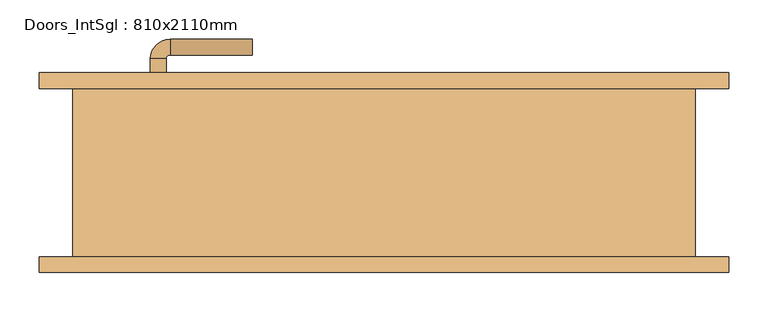
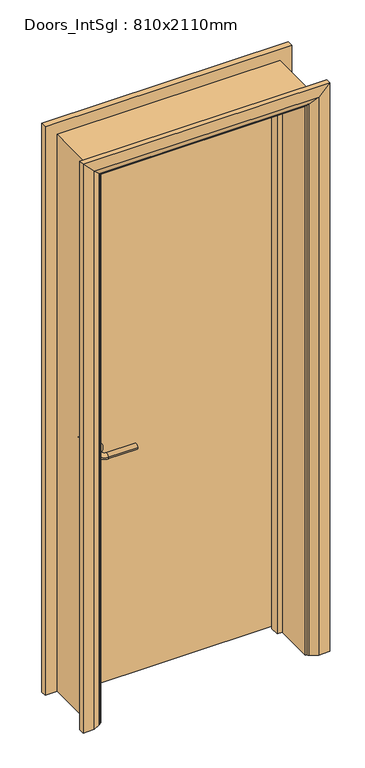
"""IFC4 building model written with IfcOpenShell, lengths in millimetres: door geometry, Doors_IntSgl : 810x2110mm."""

from ifc_helpers import new_model, si_unit, point, frame, frame_2d, origin, place, context, project, spatial, polyline, circle_curve, ellipse_curve, trimmed, segment, composite_curve, outline, extrude, faceted_brep, source, transform, mapped, element, save
from ifc_brep_helpers import plane_surface, cylinder_surface, revolved_surface, advanced_brep


def doors_intsgl_810x2110mm_df607d29(model_context):
    return source(origin(), model_context, "Body", "SolidModel", [
        advanced_brep(
        [(-298.0, 61.5, 900.0), (-278.0, 61.5, 900.0), (-278.0, 31.5, 900.0), (-298.0, 31.5, 900.0), (-273.0, 26.5, 900.0), (-273.0, 6.5, 900.0), (-168.0, 6.5, 900.0), (-168.0, 26.5, 900.0)],
        [
            (0, 1, circle_curve(frame((-288.0, 61.5, 900.0), z_axis=(0.0, 1.0, 0.0), x_axis=(1.0, 0.0, 0.0)), 10.0)),
            (1, 0, circle_curve(frame((-288.0, 61.5, 900.0), z_axis=(0.0, 1.0, 0.0), x_axis=(1.0, 0.0, 0.0)), 10.0)),
            (1, 2),
            (2, 3, circle_curve(frame((-288.0, 31.5, 900.0), z_axis=(0.0, 1.0, 0.0), x_axis=(1.0, 0.0, 0.0)), 10.0)),
            (3, 0),
            (3, 2, circle_curve(frame((-288.0, 31.5, 900.0), z_axis=(0.0, 1.0, 0.0), x_axis=(1.0, 0.0, 0.0)), 10.0)),
            (4, 5, circle_curve(frame((-273.0, 16.5, 900.0), z_axis=(-1.0, 0.0, 0.0), x_axis=(0.0, 1.0, 0.0)), 10.0)),
            (5, 3, circle_curve(frame((-273.0, 31.5, 900.0), z_axis=(0.0, 0.0, -1.0), x_axis=(-1.0, 0.0, 0.0)), 25.0)),
            (2, 4, circle_curve(frame((-273.0, 31.5, 900.0), z_axis=(0.0, 0.0, 1.0), x_axis=(-1.0, 0.0, 0.0)), 5.0)),
            (5, 4, circle_curve(frame((-273.0, 16.5, 900.0), z_axis=(-1.0, 0.0, 0.0), x_axis=(0.0, 1.0, 0.0)), 10.0)),
            (6, 7, circle_curve(frame((-168.0, 16.5, 900.0), z_axis=(1.0, 0.0, 0.0), x_axis=(0.0, 1.0, 0.0)), 10.0)),
            (7, 6, circle_curve(frame((-168.0, 16.5, 900.0), z_axis=(1.0, 0.0, 0.0), x_axis=(0.0, 1.0, 0.0)), 10.0)),
            (4, 7),
            (6, 5),
        ],
        [
            plane_surface(frame((-288.0, 61.5, 900.0), z_axis=(0.0, 1.0, 0.0), x_axis=(0.0, 0.0, 1.0))),
            cylinder_surface(frame((-288.0, 61.5, 900.0), z_axis=(0.0, 1.0, 0.0), x_axis=(1.0, 0.0, 0.0)), 10.0),
            revolved_surface(trimmed(ellipse_curve(frame((-288.0, 31.5, 900.0), z_axis=(0.0, -1.0, 0.0), x_axis=(1.0, 0.0, 0.0)), 10.0, 10.0), [point((-298.0, 31.5, 900.0))], [point((-278.0, 31.5, 900.0))], True, "CARTESIAN"), (-273.0, 31.5, 900.0), (0.0, 0.0, -1.0)),
            revolved_surface(trimmed(ellipse_curve(frame((-288.0, 31.5, 900.0), z_axis=(0.0, -1.0, 0.0), x_axis=(1.0, 0.0, 0.0)), 10.0, 10.0), [point((-278.0, 31.5, 900.0))], [point((-298.0, 31.5, 900.0))], True, "CARTESIAN"), (-273.0, 31.5, 900.0), (0.0, 0.0, -1.0)),
            plane_surface(frame((-168.0, 16.5, 900.0), z_axis=(1.0, 0.0, 0.0), x_axis=(0.0, 0.0, 1.0))),
            cylinder_surface(frame((-273.0, 16.5, 900.0), z_axis=(-1.0, 0.0, 0.0), x_axis=(0.0, 1.0, 0.0)), 10.0),
        ],
        [
            (0, [[1, 2]]),
            (1, [[3, 4, 5, -2]]),
            (1, [[-5, 6, -3, -1]]),
            (2, [[7, 8, -4, 9]]),
            (3, [[10, -9, -6, -8]]),
            (4, [[11, 12]]),
            (5, [[13, -11, 14, -7]]),
            (5, [[-14, -12, -13, -10]]),
        ],
    ),
        extrude(outline(composite_curve([segment(trimmed(circle_curve(frame_2d((900.0, -290.5)), 30.0), [point((900.0, -320.5))], [point((900.0, -260.5))], False, "CARTESIAN"), True, "CONTINUOUS"), segment(trimmed(circle_curve(frame_2d((900.0, -290.5)), 30.0), [point((900.0, -260.5))], [point((900.0, -320.5))], False, "CARTESIAN"), True, "CONTINUOUS")], self_intersect=False)), frame((0.0, 61.5, 0.0), z_axis=(0.0, 1.0, 0.0), x_axis=(0.0, 0.0, 1.0)), (0.0, 0.0, 1.0), 8.0),
        advanced_brep(
        [(-298.0, 115.5, 900.0), (-278.0, 115.5, 900.0), (-298.0, 145.5, 900.0), (-278.0, 145.5, 900.0), (-273.0, 150.5, 900.0), (-273.0, 170.5, 900.0), (-168.0, 170.5, 900.0), (-168.0, 150.5, 900.0)],
        [
            (0, 1, circle_curve(frame((-288.0, 115.5, 900.0), z_axis=(0.0, -1.0, 0.0), x_axis=(1.0, 0.0, 0.0)), 10.0)),
            (1, 0, circle_curve(frame((-288.0, 115.5, 900.0), z_axis=(0.0, -1.0, 0.0), x_axis=(1.0, 0.0, 0.0)), 10.0)),
            (0, 2),
            (2, 3, circle_curve(frame((-288.0, 145.5, 900.0), z_axis=(0.0, -1.0, 0.0), x_axis=(1.0, 0.0, 0.0)), 10.0)),
            (3, 1),
            (3, 2, circle_curve(frame((-288.0, 145.5, 900.0), z_axis=(0.0, -1.0, 0.0), x_axis=(1.0, 0.0, 0.0)), 10.0)),
            (4, 3, circle_curve(frame((-273.0, 145.5, 900.0), z_axis=(0.0, 0.0, 1.0), x_axis=(-1.0, 0.0, 0.0)), 5.0)),
            (2, 5, circle_curve(frame((-273.0, 145.5, 900.0), z_axis=(0.0, 0.0, -1.0), x_axis=(-1.0, 0.0, 0.0)), 25.0)),
            (5, 4, circle_curve(frame((-273.0, 160.5, 900.0), z_axis=(-1.0, 0.0, 0.0), x_axis=(0.0, -1.0, 0.0)), 10.0)),
            (4, 5, circle_curve(frame((-273.0, 160.5, 900.0), z_axis=(-1.0, 0.0, 0.0), x_axis=(0.0, -1.0, 0.0)), 10.0)),
            (6, 7, circle_curve(frame((-168.0, 160.5, 900.0), z_axis=(1.0, 0.0, 0.0), x_axis=(0.0, -1.0, 0.0)), 10.0)),
            (7, 6, circle_curve(frame((-168.0, 160.5, 900.0), z_axis=(1.0, 0.0, 0.0), x_axis=(0.0, -1.0, 0.0)), 10.0)),
            (5, 6),
            (7, 4),
        ],
        [
            plane_surface(frame((-288.0, 115.5, 900.0), z_axis=(0.0, -1.0, 0.0), x_axis=(0.0, 0.0, 1.0))),
            cylinder_surface(frame((-288.0, 115.5, 900.0), z_axis=(0.0, -1.0, 0.0), x_axis=(1.0, 0.0, 0.0)), 10.0),
            revolved_surface(trimmed(ellipse_curve(frame((-288.0, 145.5, 900.0), z_axis=(0.0, -1.0, 0.0), x_axis=(1.0, 0.0, 0.0)), 10.0, 10.0), [point((-298.0, 145.5, 900.0))], [point((-278.0, 145.5, 900.0))], True, "CARTESIAN"), (-273.0, 145.5, 900.0), (0.0, 0.0, -1.0)),
            revolved_surface(trimmed(ellipse_curve(frame((-288.0, 145.5, 900.0), z_axis=(0.0, -1.0, 0.0), x_axis=(1.0, 0.0, 0.0)), 10.0, 10.0), [point((-278.0, 145.5, 900.0))], [point((-298.0, 145.5, 900.0))], True, "CARTESIAN"), (-273.0, 145.5, 900.0), (0.0, 0.0, -1.0)),
            plane_surface(frame((-168.0, 160.5, 900.0), z_axis=(1.0, 0.0, 0.0), x_axis=(0.0, 0.0, 1.0))),
            cylinder_surface(frame((-273.0, 160.5, 900.0), z_axis=(-1.0, 0.0, 0.0), x_axis=(0.0, -1.0, 0.0)), 10.0),
        ],
        [
            (0, [[1, 2]]),
            (1, [[-1, 3, 4, 5]]),
            (1, [[-2, -5, 6, -3]]),
            (2, [[7, -4, 8, 9]]),
            (3, [[-8, -6, -7, 10]]),
            (4, [[11, 12]]),
            (5, [[-9, 13, -12, 14]]),
            (5, [[-10, -14, -11, -13]]),
        ],
    ),
        extrude(outline(composite_curve([segment(trimmed(circle_curve(frame_2d((900.0, -290.5)), 30.0), [point((900.0, -320.5))], [point((900.0, -260.5))], False, "CARTESIAN"), True, "CONTINUOUS"), segment(trimmed(circle_curve(frame_2d((900.0, -290.5)), 30.0), [point((900.0, -260.5))], [point((900.0, -320.5))], False, "CARTESIAN"), True, "CONTINUOUS")], self_intersect=False)), frame((0.0, 107.5, 0.0), z_axis=(0.0, 1.0, 0.0), x_axis=(0.0, 0.0, 1.0)), (0.0, 0.0, 1.0), 8.0),
        extrude(outline(polyline([(363.0, 69.5), (-363.0, 69.5), (-363.0, 107.5), (363.0, 107.5), (363.0, 69.5)])), frame((0.0, 0.0, 8.0), z_axis=(0.0, 0.0, 1.0), x_axis=(1.0, 0.0, 0.0)), (0.0, 0.0, 1.0), 2060.0),
        advanced_brep(
        [(440.0, 127.5, 0.0), (440.0, 107.5, 0.0), (370.0, 107.5, 0.0), (374.0, 113.5, 0.0), (400.0, 127.5, 0.0), (440.0, 127.5, 2145.0), (440.0, 107.5, 2145.0), (-440.0, 107.5, 2145.0), (-440.0, 107.5, 0.0), (-370.0, 107.5, 0.0), (-370.0, 107.5, 2075.0), (370.0, 107.5, 2075.0), (374.0, 113.5, 2079.0), (400.0, 127.5, 2105.0), (-400.0, 127.5, 2105.0), (-400.0, 127.5, 0.0), (-440.0, 127.5, 0.0), (-440.0, 127.5, 2145.0), (-374.0, 113.5, 2079.0), (-374.0, 113.5, 0.0)],
        [
            (0, 1),
            (1, 2),
            (2, 3, circle_curve(frame((378.0, 106.5, 0.0), z_axis=(0.0, 0.0, -1.0), x_axis=(1.0, 0.0, 0.0)), 8.0622577)),
            (3, 4),
            (4, 0),
            (0, 5),
            (5, 6),
            (6, 1),
            (6, 7),
            (7, 8),
            (8, 9),
            (9, 10),
            (10, 11),
            (11, 2),
            (11, 12, ellipse_curve(frame((378.0, 106.5, 2083.0), z_axis=(0.7071067811865475, 0.0, -0.7071067811865475), x_axis=(-0.7071067811865474, 0.0, -0.7071067811865476)), 11.4017543, 8.0622577)),
            (12, 3),
            (12, 13),
            (13, 4),
            (13, 14),
            (14, 15),
            (15, 16),
            (16, 17),
            (17, 5),
            (17, 7),
            (10, 18, ellipse_curve(frame((-378.0, 106.5, 2083.0), z_axis=(0.7071067811865475, 0.0, 0.7071067811865475), x_axis=(0.7071067811865476, 0.0, -0.7071067811865474)), 11.4017543, 8.0622577)),
            (18, 12),
            (18, 14),
            (15, 19),
            (19, 9, circle_curve(frame((-378.0, 106.5, 0.0), z_axis=(0.0, 0.0, -1.0), x_axis=(-1.0, 0.0, 0.0)), 8.0622577)),
            (8, 16),
            (19, 18),
        ],
        [
            plane_surface(frame((370.0, 107.5, 0.0), z_axis=(0.0, 0.0, -1.0), x_axis=(0.0, -1.0, 0.0))),
            plane_surface(frame((440.0, 127.5, 0.0), z_axis=(1.0, 0.0, 0.0), x_axis=(0.0, 0.0, 1.0))),
            plane_surface(frame((440.0, 107.5, 0.0), z_axis=(0.0, -1.0, 0.0), x_axis=(0.0, 0.0, 1.0))),
            cylinder_surface(frame((378.0, 106.5, 0.0), z_axis=(0.0, 0.0, -1.0), x_axis=(1.0, 0.0, 0.0)), 8.0622577),
            plane_surface(frame((374.0, 113.5, 0.0), z_axis=(-0.4740998230350126, 0.880471099922178, 0.0), x_axis=(0.0, 0.0, 1.0))),
            plane_surface(frame((400.0, 127.5, 0.0), z_axis=(0.0, 1.0, 0.0), x_axis=(0.0, 0.0, 1.0))),
            plane_surface(frame((440.0, 127.5, 2145.0), z_axis=(0.0, 0.0, 1.0), x_axis=(-1.0, 0.0, 0.0))),
            cylinder_surface(frame((370.0, 106.5, 2083.0), z_axis=(1.0, 0.0, 0.0), x_axis=(0.0, 0.0, 1.0)), 8.0622577),
            plane_surface(frame((374.0, 113.5, 2079.0), z_axis=(0.0, 0.8804710999221764, -0.4740998230350154), x_axis=(-1.0, 0.0, 0.0))),
            plane_surface(frame((-370.0, 107.5, 0.0), z_axis=(0.0, 0.0, -1.0), x_axis=(0.0, -1.0, 0.0))),
            plane_surface(frame((-440.0, 127.5, 2145.0), z_axis=(-1.0, 0.0, 0.0), x_axis=(0.0, 0.0, -1.0))),
            cylinder_surface(frame((-378.0, 106.5, 2075.0), z_axis=(0.0, 0.0, 1.0), x_axis=(-1.0, 0.0, 0.0)), 8.0622577),
            plane_surface(frame((-374.0, 113.5, 2079.0), z_axis=(0.47409982303501824, 0.8804710999221749, 0.0), x_axis=(0.0, 0.0, -1.0))),
        ],
        [
            (0, [[1, 2, 3, 4, 5]]),
            (1, [[-1, 6, 7, 8]]),
            (2, [[-2, -8, 9, 10, 11, 12, 13, 14]]),
            (3, [[-3, -14, 15, 16]]),
            (4, [[-4, -16, 17, 18]]),
            (5, [[-5, -18, 19, 20, 21, 22, 23, -6]]),
            (6, [[-7, -23, 24, -9]]),
            (7, [[-15, -13, 25, 26]]),
            (8, [[-17, -26, 27, -19]]),
            (9, [[-21, 28, 29, -11, 30]]),
            (10, [[-24, -22, -30, -10]]),
            (11, [[-25, -12, -29, 31]]),
            (12, [[-27, -31, -28, -20]]),
        ],
    ),
        extrude(outline(polyline([(0.0, -365.0), (0.0, -346.0), (2051.0, -346.0), (2051.0, 346.0), (0.0, 346.0), (0.0, 365.0), (2070.0, 365.0), (2070.0, -365.0), (0.0, -365.0)])), frame((0.0, 35.5, 0.0), z_axis=(0.0, 1.0, 0.0), x_axis=(0.0, 0.0, 1.0)), (0.0, 0.0, 1.0), 32.0),
        advanced_brep(
        [(-440.0, -127.5, 0.0), (-440.0, -107.5, 0.0), (-370.0, -107.5, 0.0), (-374.0, -113.5, 0.0), (-400.0, -127.5, 0.0), (-440.0, -127.5, 2145.0), (-440.0, -107.5, 2145.0), (-370.0, -107.5, 2075.0), (-374.0, -113.5, 2079.0), (-400.0, -127.5, 2105.0), (440.0, -127.5, 2145.0), (440.0, -107.5, 2145.0), (370.0, -107.5, 2075.0), (374.0, -113.5, 2079.0), (400.0, -127.5, 2105.0), (440.0, -127.5, 0.0), (400.0, -127.5, 0.0), (374.0, -113.5, 0.0), (370.0, -107.5, 0.0), (440.0, -107.5, 0.0)],
        [
            (0, 1),
            (1, 2),
            (2, 3, circle_curve(frame((-378.0, -106.5, 0.0), z_axis=(0.0, 0.0, -1.0), x_axis=(-1.0, 0.0, 0.0)), 8.0622577)),
            (3, 4),
            (4, 0),
            (0, 5),
            (5, 6),
            (6, 1),
            (6, 7),
            (7, 2),
            (7, 8, ellipse_curve(frame((-378.0, -106.5, 2083.0), z_axis=(-0.7071067811865475, 0.0, -0.7071067811865475), x_axis=(0.7071067811865474, 0.0, -0.7071067811865476)), 11.4017543, 8.0622577)),
            (8, 3),
            (8, 9),
            (9, 4),
            (9, 5),
            (5, 10),
            (10, 11),
            (11, 6),
            (11, 12),
            (12, 7),
            (12, 13, ellipse_curve(frame((378.0, -106.5, 2083.0), z_axis=(-0.7071067811865475, 0.0, 0.7071067811865475), x_axis=(-0.7071067811865476, 0.0, -0.7071067811865474)), 11.4017543, 8.0622577)),
            (13, 8),
            (13, 14),
            (14, 9),
            (14, 10),
            (15, 16),
            (16, 17),
            (17, 18, circle_curve(frame((378.0, -106.5, 0.0), z_axis=(0.0, 0.0, -1.0), x_axis=(1.0, 0.0, 0.0)), 8.0622577)),
            (18, 19),
            (19, 15),
            (10, 15),
            (19, 11),
            (18, 12),
            (17, 13),
            (16, 14),
        ],
        [
            plane_surface(frame((-370.0, -180.3010989, 0.0), z_axis=(0.0, 0.0, -1.0), x_axis=(1.0, 0.0, 0.0))),
            plane_surface(frame((-440.0, -127.5, 0.0), z_axis=(-1.0, 0.0, 0.0), x_axis=(0.0, 0.0, 1.0))),
            plane_surface(frame((-440.0, -107.5, 0.0), z_axis=(0.0, 1.0, 0.0), x_axis=(0.0, 0.0, 1.0))),
            cylinder_surface(frame((-378.0, -106.5, 0.0), z_axis=(0.0, 0.0, -1.0), x_axis=(-1.0, 0.0, 0.0)), 8.0622577),
            plane_surface(frame((-374.0, -113.5, 0.0), z_axis=(0.4740998230350183, -0.8804710999221749, 0.0), x_axis=(0.0, 0.0, 1.0))),
            plane_surface(frame((-400.0, -127.5, 0.0), z_axis=(0.0, -1.0, 0.0), x_axis=(0.0, 0.0, 1.0))),
            plane_surface(frame((-440.0, -127.5, 2145.0), z_axis=(0.0, 0.0, 1.0), x_axis=(1.0, 0.0, 0.0))),
            plane_surface(frame((-440.0, -107.5, 2145.0), z_axis=(0.0, 1.0, 0.0), x_axis=(1.0, 0.0, 0.0))),
            cylinder_surface(frame((-370.0, -106.5, 2083.0), z_axis=(-1.0, 0.0, 0.0), x_axis=(0.0, 0.0, 1.0)), 8.0622577),
            plane_surface(frame((-374.0, -113.5, 2079.0), z_axis=(0.0, -0.8804710999221749, -0.4740998230350183), x_axis=(1.0, 0.0, 0.0))),
            plane_surface(frame((-400.0, -127.5, 2105.0), z_axis=(0.0, -1.0, 0.0), x_axis=(1.0, 0.0, 0.0))),
            plane_surface(frame((370.0, -180.3010989, 0.0), z_axis=(0.0, 0.0, -1.0), x_axis=(-1.0, 0.0, 0.0))),
            plane_surface(frame((440.0, -127.5, 2145.0), z_axis=(1.0, 0.0, 0.0), x_axis=(0.0, 0.0, -1.0))),
            plane_surface(frame((440.0, -107.5, 2145.0), z_axis=(0.0, 1.0, 0.0), x_axis=(0.0, 0.0, -1.0))),
            cylinder_surface(frame((378.0, -106.5, 2075.0), z_axis=(0.0, 0.0, 1.0), x_axis=(1.0, 0.0, 0.0)), 8.0622577),
            plane_surface(frame((374.0, -113.5, 2079.0), z_axis=(-0.4740998230350183, -0.8804710999221749, 0.0), x_axis=(0.0, 0.0, -1.0))),
            plane_surface(frame((400.0, -127.5, 2105.0), z_axis=(0.0, -1.0, 0.0), x_axis=(0.0, 0.0, -1.0))),
        ],
        [
            (0, [[1, 2, 3, 4, 5]]),
            (1, [[-1, 6, 7, 8]]),
            (2, [[-2, -8, 9, 10]]),
            (3, [[-3, -10, 11, 12]]),
            (4, [[-4, -12, 13, 14]]),
            (5, [[-5, -14, 15, -6]]),
            (6, [[-7, 16, 17, 18]]),
            (7, [[-9, -18, 19, 20]]),
            (8, [[-11, -20, 21, 22]]),
            (9, [[-13, -22, 23, 24]]),
            (10, [[-15, -24, 25, -16]]),
            (11, [[26, 27, 28, 29, 30]]),
            (12, [[-17, 31, -30, 32]]),
            (13, [[-19, -32, -29, 33]]),
            (14, [[-21, -33, -28, 34]]),
            (15, [[-23, -34, -27, 35]]),
            (16, [[-25, -35, -26, -31]]),
        ],
    ),
        faceted_brep([(-365.0, 107.5, 0.0), (-365.0, -107.5, 0.0), (-397.0, -107.5, 0.0), (-397.0, 107.5, 0.0), (-365.0, 107.5, 2070.0), (-365.0, -107.5, 2070.0), (-397.0, -107.5, 2102.0), (-397.0, 107.5, 2102.0), (365.0, 107.5, 2070.0), (365.0, -107.5, 2070.0), (397.0, -107.5, 2102.0), (397.0, 107.5, 2102.0), (365.0, 107.5, 0.0), (397.0, 107.5, 0.0), (397.0, -107.5, 0.0), (365.0, -107.5, 0.0)], [[[0, 1, 2, 3]], [[1, 0, 4, 5]], [[2, 1, 5, 6]], [[3, 2, 6, 7]], [[0, 3, 7, 4]], [[5, 4, 8, 9]], [[6, 5, 9, 10]], [[7, 6, 10, 11]], [[4, 7, 11, 8]], [[12, 13, 14, 15]], [[9, 8, 12, 15]], [[10, 9, 15, 14]], [[11, 10, 14, 13]], [[8, 11, 13, 12]]]),
    ])


if __name__ == "__main__":
    model = new_model("IFC4")
    model_context = context("Model", 3, world=origin())
    ifc_project = project(units=[si_unit("LENGTHUNIT", "METRE", prefix="MILLI")], contexts=[model_context])
    site = spatial("IfcSite", under=ifc_project)
    building = spatial("IfcBuilding", under=site)
    placement = place(None, origin())
    doors_intsgl_810x2110mm_shape = doors_intsgl_810x2110mm_df607d29(model_context)
    element("IfcDoor", 1, ObjectType="Doors_IntSgl : 810x2110mm", at=placement, inside=building, context=model_context, shape_type="MappedRepresentation", body=[
        mapped(doors_intsgl_810x2110mm_shape, transform((0.0, 0.0, 0.0), x_axis=(1.0, 0.0, 0.0), y_axis=(0.0, 1.0, 0.0), z_axis=(0.0, 0.0, 1.0))),
    ])
    save(model, "model.ifc")

# Revit data of these elements
# Type "Doors_IntSgl : 810x2110mm"
#   Construction Type Id = "MDOOR"
#   Type Mark = "42"
#   Type Comments = "Internal Single"
#   Operation = "SingleSwingRight"
#   Manufacturer = "Revit"
#   Keynote = "L20"
#   Description = "Internal Single Door"
#   Analytic Construction = "Metal"
#   UnderCut = 8 mm
#   Tolerance = 2 mm
#   Thickness = 38 mm
#   Thermal Resistance (R) = 0.270117 (m²·K)/W
#   Structural Tolerance = 8 mm
#   StopDepth = 32 mm
#   Stop Thickness = 19 mm
#   Rough Width = 810 mm
#   Rough Height = 2110 mm
#   Height to Top Lock Rail = 1000 mm
#   Heat Transfer Coefficient (U) = 3.7021 W/(m²·K)
#   Handle Z Distance = 900 mm
#   Handle X Distance = 75 mm
#   Frame Thickness = 32 mm
#   Door Panel Width = 726 mm
#   Door Panel Thickness = 38 mm
#   Door Panel Offset = 0 mm
#   Height = 2110 mm
#   Width = 810 mm
#   Door Panel Height = 2060 mm
#   Architrave Setback = 5 mm
#   Define Thermal Properties by = 1
#   Vis - Ironmongery = yes
#   Material Ironmongery = Door - Handle
#   Material Frame = Door - Frame/Mullion (1)
#   Material Door = Door - Panel
#   Material Architrave = Door - Architrave
#   Visual Light Transmittance = 0
#   Solar Heat Gain Coefficient = 0
#   Function = (empty or 0)
#   Wall Closure = (empty or 0)
# Element 1 (IfcDoor, "Doors_IntSgl : 810x2110mm")
#   Materials on its faces: "Door - Architrave", "Door - Handle", "Door - Frame/Mullion (1)", "Door - Panel"
# Materials
#   "Door - Handle": colour RGB 0 0 0, transparency 0, Keynote = "P21", Cost = 0
#   "Door - Frame/Mullion (1)": class "Wood", colour RGB 212 179 113, transparency 0, Keynote = "L20", Cost = 0
#   "Door - Panel": class "Wood", colour RGB 210 159 95, transparency 0, Keynote = "L20", Cost = 0
#   "Door - Architrave": class "Wood", colour RGB 154 90 5, transparency 0, Keynote = "P20", Cost = 0
